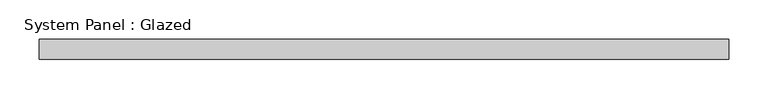
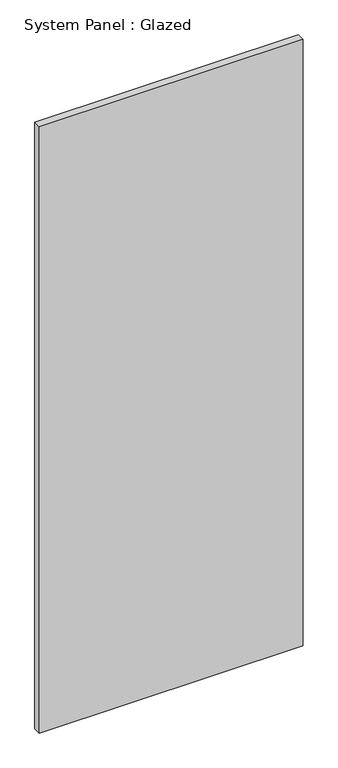
"""IFC4 building model written with IfcOpenShell, lengths in millimetres: plate geometry, System Panel : Glazed."""

from ifc_helpers import new_model, si_unit, origin, origin_with_axes, place, context, project, spatial, polyline, outline, extrude, source, transform, mapped, element, save


def system_panel_glazed_303585a9(model_context):
    return source(origin(), model_context, "Body", "SweptSolid", [
        extrude(outline(polyline([(438.15, 19.05), (-438.15, 19.05), (-438.15, 44.45), (438.15, 44.45), (438.15, 19.05)])), origin_with_axes(), (0.0, 0.0, 1.0), 2127.3645985),
    ])


if __name__ == "__main__":
    model = new_model("IFC4")
    model_context = context("Model", 3, world=origin())
    ifc_project = project(units=[si_unit("LENGTHUNIT", "METRE", prefix="MILLI")], contexts=[model_context])
    site = spatial("IfcSite", under=ifc_project)
    building = spatial("IfcBuilding", under=site)
    placement = place(None, origin())
    system_panel_glazed_shape = system_panel_glazed_303585a9(model_context)
    element("IfcPlate", 1, ObjectType="System Panel : Glazed", at=placement, inside=building, context=model_context, shape_type="MappedRepresentation", body=[
        mapped(system_panel_glazed_shape, transform((0.0, 0.0, 0.0), x_axis=(1.0, 0.0, 0.0), y_axis=(0.0, 1.0, 0.0), z_axis=(0.0, 0.0, 1.0))),
    ])
    save(model, "model.ifc")

# Revit data of these elements
# Type "System Panel : Glazed"
#   Construction Type Id = "GSP4R"
#   Analytic Construction = "1/8 in Pilkington single glazing"
#   Visual Light Transmittance = 0.9
#   Solar Heat Gain Coefficient = 0.86
#   Heat Transfer Coefficient (U) = 1.18115 BTU/(h·ft²·°F)
#   Define Thermal Properties by = 1
# Element 1 (IfcPlate, "System Panel : Glazed")
#   Materials on its faces: "Glass"
# Materials
#   "Glass": class "Glass", colour RGB 0 128 192, transparency 0.75, Description = "Soda Lime Glass", Cost = 0
